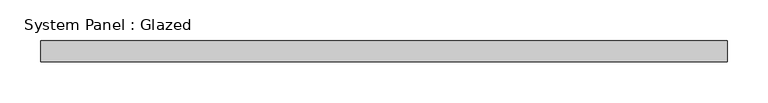
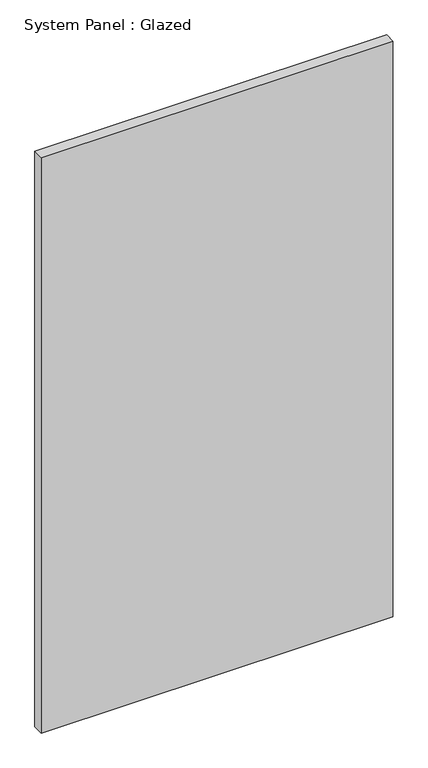
"""IFC4 building model written with IfcOpenShell, lengths in millimetres: plate geometry, System Panel : Glazed."""

from ifc_helpers import new_model, si_unit, origin, origin_with_axes, place, context, project, spatial, polyline, outline, extrude, source, transform, mapped, element, save


def system_panel_glazed_f96bbed7(model_context):
    return source(origin(), model_context, "Body", "SweptSolid", [
        extrude(outline(polyline([(419.1, 19.05), (-419.1, 19.05), (-419.1, 44.45), (419.1, 44.45), (419.1, 19.05)])), origin_with_axes(), (0.0, 0.0, 1.0), 1449.4289848),
    ])


if __name__ == "__main__":
    model = new_model("IFC4")
    model_context = context("Model", 3, world=origin())
    ifc_project = project(units=[si_unit("LENGTHUNIT", "METRE", prefix="MILLI")], contexts=[model_context])
    site = spatial("IfcSite", under=ifc_project)
    building = spatial("IfcBuilding", under=site)
    placement = place(None, origin())
    system_panel_glazed_shape = system_panel_glazed_f96bbed7(model_context)
    element("IfcPlate", 1, ObjectType="System Panel : Glazed", at=placement, inside=building, context=model_context, shape_type="MappedRepresentation", body=[
        mapped(system_panel_glazed_shape, transform((0.0, 0.0, 0.0), x_axis=(1.0, 0.0, 0.0), y_axis=(0.0, 1.0, 0.0), z_axis=(0.0, 0.0, 1.0))),
    ])
    save(model, "model.ifc")

# Revit data of these elements
# Type "System Panel : Glazed"
#   Construction Type Id = "GSP4R"
#   Analytic Construction = "1/8 in Pilkington single glazing"
#   Visual Light Transmittance = 0.9
#   Solar Heat Gain Coefficient = 0.86
#   Heat Transfer Coefficient (U) = 1.18115 BTU/(h·ft²·°F)
#   Define Thermal Properties by = 1
# Element 1 (IfcPlate, "System Panel : Glazed")
#   Materials on its faces: "Glass"
# Materials
#   "Glass": class "Glass", colour RGB 0 128 192, transparency 0.75, Description = "Soda Lime Glass", Cost = 0
